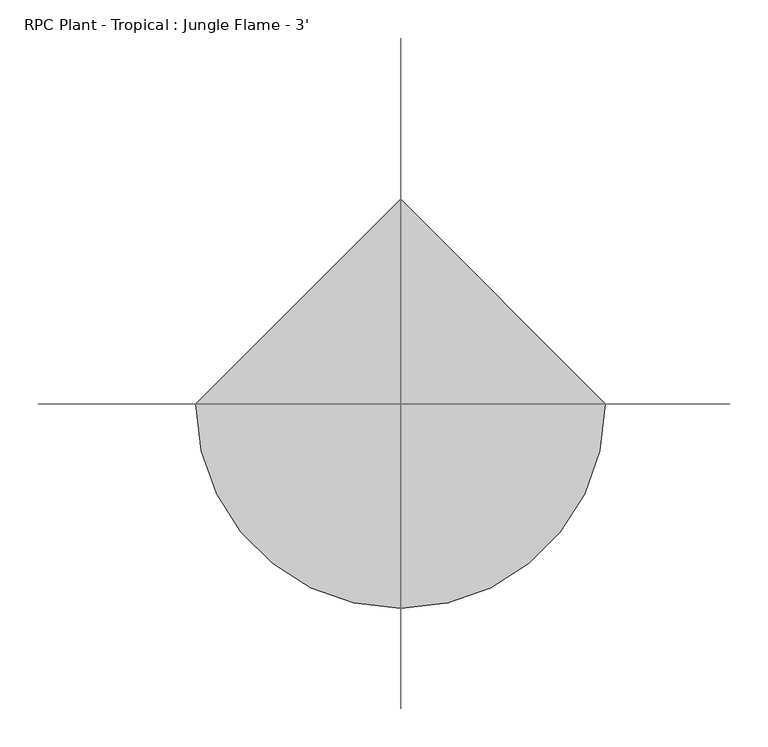
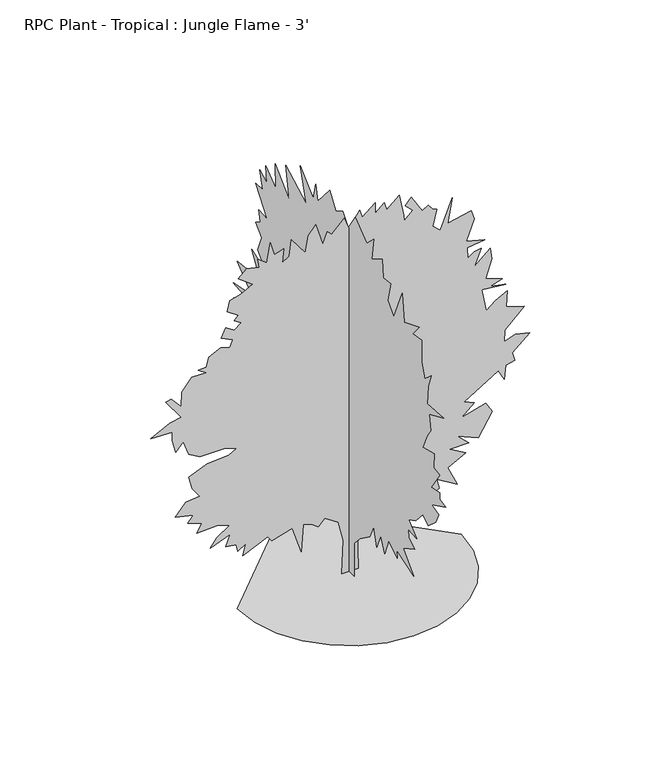
"""IFC4 building model written with IfcOpenShell, lengths in millimetres: geographic element geometry, RPC Plant - Tropical : Jungle Flame - 3'."""

from ifc_helpers import new_model, si_unit, origin, place, context, project, spatial, triangles, source, transform, mapped, element, save


def rpc_plant_tropical_jungle_flame_3_9c4808c2(model_context):
    return source(origin(), model_context, "Body", "Tessellation", [
        triangles([(-268.0952273, 0.0, 4.64e-05), (-261.0086141, -61.4296216, 4.64e-05), (-240.8232365, -117.8430704, 4.64e-05), (-209.155511, -167.6236892, 4.64e-05), (-167.6236892, -209.1557472, 4.64e-05), (-117.8430704, -240.8232365, 4.64e-05), (-61.4296216, -261.0086141, 4.64e-05), (1.17e-05, -268.0952273, 4.64e-05), (61.4296216, -261.0086141, 4.64e-05), (117.8430704, -240.8232365, 4.64e-05), (167.6236892, -209.155511, 4.64e-05), (209.1557472, -167.6236892, 4.64e-05), (240.8232365, -117.8430704, 4.64e-05), (261.0086141, -61.4296216, 4.64e-05), (268.0952273, 2.34e-05, 4.64e-05), (-3.52e-05, 268.0952273, 4.64e-05), (-1.48e-05, -20.1101483, 4.49e-05), (-1.23e-05, -20.1680527, 84.1033148), (-1.26e-05, -43.4307974, 109.1553558), (-1.36e-05, -84.5877148, 139.5758464), (-1.33e-05, -102.4820622, 175.3643141), (-1.52e-05, -115.0079782, 130.6286726), (-1.47e-05, -131.1128455, 169.9961098), (-1.65e-05, -147.2177128, 134.2074059), (-1.6e-05, -163.3225891, 177.1537943), (-1.83e-05, -199.111284, 153.8912426), (-1.76e-05, -197.3218038, 173.5750701), (-2.14e-05, -267.1099495, 150.3122731), (-1.81e-05, -224.163334, 195.0481417), (-1.95e-05, -270.6875473, 220.1001918), (-1.79e-05, -245.6375502, 234.4155789), (-1.73e-05, -243.8476158, 254.100333), (-1.89e-05, -279.6349481, 252.3103987), (-1.66e-05, -247.4252136, 280.9402645), (-1.75e-05, -276.0573685, 295.2574684), (-1.78e-05, -304.6872162, 327.4672211), (-1.92e-05, -327.9495681, 314.9399334), (-1.98e-05, -358.3716574, 341.782154), (-1.95e-05, -370.8966559, 368.6220855), (-1.8e-05, -342.2667901, 375.7818229), (-1.97e-05, -399.5287745, 404.4116887), (-1.85e-05, -374.4765246, 409.7792027), (-1.8e-05, -374.4765246, 425.8840699), (-1.67e-05, -340.4768558, 418.7266216), (-1.67e-05, -374.4765246, 470.6210921), (-1.54e-05, -349.4242384, 474.1987081), (-1.44e-05, -351.2141727, 509.9883113), (-1.27e-05, -304.6872162, 499.250958), (-1.23e-05, -322.5820178, 538.6181771), (-1.23e-05, -336.8969507, 560.0928474), (-1.09e-05, -331.5294368, 597.6701323), (-1.28e-05, -390.5813919, 624.5123165), (-9.9e-06, -322.5820178, 619.1448389), (-8.7e-06, -327.9495681, 667.4594044), (-8.2e-06, -338.6868851, 699.6691389), (-7.7e-06, -311.8447008, 676.4045706), (-6.1e-06, -299.3197022, 710.4042395), (-4.5e-06, -299.3197022, 765.8762896), (-3.1e-06, -263.5300808, 760.5087393), (-3.3e-06, -290.3722833, 792.7184738), (-1.2e-06, -227.7422944, 767.6662239), (1.2e-06, -218.7951116, 835.6655617), (3e-07, -184.7958969, 755.1412617), (2.2e-06, -159.7438468, 781.9811932), (3.2e-06, -172.2697537, 832.085693), (4.4e-06, -141.8494994, 828.5081497), (5.9e-06, -136.4810589, 871.4529121), (7.1e-06, -93.5348885, 846.4006622), (8.4e-06, -100.692582, 900.0851034), (8.9e-06, -72.0615762, 873.2428465), (1.21e-05, -25.5364477, 910.8201313), (1.2e-05, 3.0945581, 866.0853619), (1.39e-05, 26.3571235, 894.7152277), (1.47e-05, 54.9881316, 878.6103968), (1.69e-05, 80.0401726, 914.4), (1.74e-05, 130.1442636, 857.1380156), (1.89e-05, 139.0914373, 894.7152277), (1.81e-05, 149.8281003, 851.7704653), (2.2e-05, 203.5109246, 901.8750378), (1.85e-05, 178.4588745, 821.3506651), (2.37e-05, 262.5630977, 867.8752962), (2.07e-05, 248.2458757, 789.1409306), (2.49e-05, 305.5079146, 844.6129807), (2.3e-05, 303.7202512, 783.7711275), (2.58e-05, 344.8750975, 815.980862), (2.44e-05, 341.2975179, 774.8237085), (2.62e-05, 369.9273837, 790.9285395), (2.43e-05, 357.4023851, 747.983777), (2.56e-05, 387.8221853, 746.1938427), (2.16e-05, 339.5075835, 683.564308), (2.32e-05, 373.5072524, 687.1418512), (2.22e-05, 368.1397385, 660.299667), (2.27e-05, 387.8221853, 647.7747047), (2.08e-05, 362.7698991, 622.7223822), (2.04e-05, 378.8747663, 583.3551993), (1.77e-05, 343.0874522, 547.5655961), (2.11e-05, 403.9270526, 569.0402664), (1.71e-05, 360.9799647, 499.250958), (1.89e-05, 393.1896993, 511.7782456), (2.17e-05, 462.9790077, 502.830863), (1.77e-05, 403.9270526, 454.5162249), (2.05e-05, 479.083875, 438.4113576), (1.67e-05, 396.7696043, 431.2539093), (1.57e-05, 387.8221853, 411.569137), (1.94e-05, 477.2939406, 402.6217544), (1.5e-05, 394.97967, 377.5694681), (1.44e-05, 411.0845372, 332.834735), (1.36e-05, 368.1397385, 370.4120198), (1.19e-05, 355.6124508, 334.6246694), (1.33e-05, 398.5595387, 314.9399334), (1.21e-05, 400.349473, 271.9928455), (8.7e-06, 341.2975179, 248.7305118), (1.01e-05, 384.2446057, 229.0480649), (4.9e-06, 291.1929636, 195.0481417), (6.5e-06, 341.2975179, 175.3643141), (6.7e-06, 369.9273837, 135.996886), (4.2e-06, 294.7728504, 166.4173675), (2.6e-06, 289.4030292, 121.6814898), (2.3e-06, 258.983229, 157.4702029), (0.0, 239.300764, 107.3661027), (1.6e-06, 241.0884092, 159.2594469), (1.2e-06, 228.5629746, 164.6278873), (-1.1e-06, 203.5109246, 127.0497123), (-2e-07, 205.3004047, 153.8912426), (-1.9e-06, 162.3540072, 159.2594469), (-2.4e-06, 167.7222116, 135.996886), (-3e-06, 139.0914373, 157.4702029), (-5.5e-06, 130.1442636, 89.4717553), (-5.5e-06, 74.6719592, 171.78559), (-6.4e-06, 62.1458251, 161.048927), (-7.4e-06, 37.0937796, 164.6278873), (-7.6e-06, 51.4093984, 134.2074059), (-8.5e-06, 15.6205809, 157.4702029), (-1.29e-05, 22.7783675, 4.61e-05), (-17.334692, 5.3e-05, 1.7e-06), (-13.7758477, 4.79e-05, 83.6317139), (-26.2316224, 4.54e-05, 133.4546266), (-58.2607652, 4.56e-05, 154.8074657), (-74.27534, 4.72e-05, 138.7928909), (-90.2899103, 4.72e-05, 151.2486168), (-109.863334, 4.77e-05, 156.5868811), (-115.2013712, 5.19e-05, 90.7491664), (-136.5542103, 4.89e-05, 156.5868811), (-184.5979257, 5.18e-05, 142.3517307), (-195.2742362, 5.15e-05, 156.5868811), (-253.9951796, 5.57e-05, 128.1165803), (-246.8765734, 5.37e-05, 156.5868811), (-266.4493067, 5.53e-05, 144.1311552), (-270.0086098, 5.44e-05, 161.9249273), (-294.9214242, 5.53e-05, 165.4837762), (-284.2435331, 5.31e-05, 193.954077), (-332.2884021, 5.64e-05, 174.3808894), (-316.2726645, 5.44e-05, 195.7334923), (-286.024311, 5.18e-05, 217.0863314), (-316.2726645, 5.26e-05, 225.9832084), (-364.3175517, 5.48e-05, 224.203793), (-351.8611173, 5.31e-05, 243.7767626), (-385.6687921, 5.38e-05, 256.2331607), (-373.2146467, 5.23e-05, 272.2465909), (-415.9194165, 5.36e-05, 282.9245002), (-391.0088731, 5.08e-05, 311.3943649), (-357.1989455, 4.91e-05, 314.953668), (-374.9931719, 4.84e-05, 339.8641751), (-383.8902669, 4.69e-05, 371.8933248), (-339.4047192, 4.38e-05, 391.4660763), (-287.8028362, 4.13e-05, 395.0253794), (-268.2301028, 3.98e-05, 405.7032887), (-300.2592343, 4.07e-05, 414.5980946), (-357.1989455, 4.32e-05, 414.5980946), (-383.8902669, 4.34e-05, 430.6138321), (-396.346665, 4.18e-05, 466.2022848), (-414.1408914, 4.37e-05, 446.6272442), (-423.0357336, 4.22e-05, 478.6563938), (-423.0357336, 4.09e-05, 500.0099233), (-474.6398875, 4.31e-05, 501.7884121), (-428.3758146, 3.97e-05, 524.9227558), (-401.6844933, 3.82e-05, 530.2605477), (-439.0514348, 3.68e-05, 581.8624489), (-424.8165115, 3.6e-05, 583.6409377), (-401.6844933, 3.66e-05, 556.9519054), (-399.903679, 3.44e-05, 592.5380691), (-376.7716607, 3.16e-05, 622.7887299), (-341.1854971, 3.02e-05, 621.0078793), (-360.7582486, 3.02e-05, 635.2450916), (-341.1854971, 2.93e-05, 635.2450916), (-335.8454161, 2.77e-05, 658.3771099), (-307.3755695, 2.56e-05, 672.6120695), (-286.024311, 2.51e-05, 665.4934633), (-278.905723, 2.37e-05, 683.2876534), (-305.5970444, 2.41e-05, 695.7440878), (-294.9214242, 2.23e-05, 718.8761061), (-275.3464199, 2.22e-05, 706.4197443), (-257.5521935, 2.07e-05, 718.8761061), (-275.3464199, 2.08e-05, 729.5517626), (-264.6707997, 1.97e-05, 740.2273464), (-291.3621211, 1.98e-05, 758.0216091), (-286.024311, 1.8e-05, 784.7129305), (-259.3329896, 1.64e-05, 791.8315367), (-230.8631431, 1.43e-05, 806.0664963), (-264.6707997, 1.42e-05, 832.7578176), (-245.0980664, 1.23e-05, 850.5520077), (-214.8476599, 1.14e-05, 843.4334015), (-218.4062726, 1.03e-05, 864.7869673), (-197.0536516, 1.03e-05, 848.7712297), (-188.1565384, 7e-06, 896.8161169), (-179.2596614, 8.7e-06, 863.0061167), (-156.1274069, 7.2e-06, 870.1247229), (-159.6862377, 9.4e-06, 836.3147953), (-143.6716719, 8.1e-06, 846.9927046), (-138.3334077, 5.5e-06, 886.1382076), (-104.5250607, 6.7e-06, 841.6548763), (-97.407372, 3.9e-06, 882.5811573), (-79.6133818, 1.9e-06, 903.9323977), (-63.599034, 4.4e-06, 848.7712297), (-52.922501, 2.3e-06, 877.2410763), (-42.246195, 2.5e-06, 866.5654198), (-11.9964482, -7e-07, 896.8161169), (-1.3200484, 6e-07, 868.3439449), (25.3709418, -2.7e-06, 903.9323977), (30.7089813, -1.8e-06, 884.3596825), (62.7381264, -4.7e-06, 909.2702259), (62.7381264, -3.1e-06, 882.5811573), (84.09097, -5.2e-06, 902.1538725), (89.4290072, -4.3e-06, 882.5811573), (119.6787324, -7.2e-06, 909.2702259), (130.3552609, -4.4e-06, 854.109058), (132.1346854, -3.6e-06, 839.8740984), (151.7078729, -5.6e-06, 859.449139), (133.9138827, -5.9e-06, 877.2410763), (148.1492602, -7.5e-06, 893.2568138), (174.8401455, -6.1e-06, 850.5520077), (189.0752868, -7.2e-06, 859.449139), (197.9721638, -6.9e-06, 846.9927046), (208.6487105, -7e-06, 841.6548763), (199.7515974, -4.3e-06, 802.5071932), (217.5455875, -4.1e-06, 786.4937084), (246.0147437, -9.6e-06, 857.6683611), (235.3391235, -5.5e-06, 797.1693649), (292.2811057, -8.8e-06, 809.6257267), (299.3974228, -7.7e-06, 786.4937084), (279.8246894, -3.9e-06, 736.6703688), (324.3102553, -5.1e-06, 724.2139343), (281.6031964, -2.9e-06, 718.8761061), (283.3839925, -1.4e-06, 692.1847847), (299.3974228, -2.7e-06, 702.8604412), (315.413124, -3.6e-06, 706.4197443), (299.3974228, -5e-07, 665.4934633), (336.7643643, -4.1e-06, 699.3033909), (340.3236674, -2.6e-06, 670.8312916), (326.0887442, 7e-07, 626.348033), (365.2365, -2e-07, 612.1130733), (336.7643643, 1.6e-06, 603.2159783), (374.1313422, 5e-07, 594.318847), (317.1916492, 2.5e-06, 601.4351641), (327.8672693, 5.5e-06, 544.495471), (349.2207988, 3.5e-06, 562.2896974), (377.6906453, 1.4e-06, 576.5246206), (375.9121202, 3.8e-06, 537.3768648), (418.61689, 2.8e-06, 523.1419415), (372.3528171, 7.4e-06, 478.6563938), (370.5743282, 9.2e-06, 450.1865473), (397.2633605, 7.4e-06, 460.8644566), (431.0732881, 6.5e-06, 451.9673615), (390.1470434, 1.04e-05, 416.3789088), (395.4848717, 1.14e-05, 395.0253794), (374.1313422, 1.27e-05, 389.6875511), (370.5743282, 1.48e-05, 355.8799127), (356.339405, 1.39e-05, 382.5689449), (274.4868793, 2.04e-05, 332.747858), (299.3974228, 2e-05, 322.0699851), (267.3682732, 2.3e-05, 295.3786274), (326.0887442, 1.94e-05, 311.3943649), (342.1021926, 2.03e-05, 284.7030072), (308.2945178, 2.51e-05, 229.5418393), (258.47116, 2.6e-05, 250.8953506), (285.1624995, 2.63e-05, 225.9832084), (240.6769336, 2.84e-05, 224.203793), (278.0438933, 2.8e-05, 202.8511901), (235.3391235, 3.13e-05, 179.7189175), (258.47116, 3.32e-05, 129.8957777), (208.6484744, 3.36e-05, 160.1454938), (215.7661722, 3.48e-05, 135.234042), (180.1781736, 3.73e-05, 119.2194762), (146.3698357, 3.69e-05, 149.4691923), (151.7078729, 4.11e-05, 76.5140161), (132.1346854, 3.8e-05, 142.3517307), (82.3115456, 4.26e-05, 101.425477), (91.2084316, 3.97e-05, 144.1311552), (53.8412448, 4.43e-05, 94.3080153), (43.1647072, 4.28e-05, 126.337165), (66.2969707, 3.83e-05, 185.0571818), (34.2678257, 4e-05, 179.7189175), (18.2532304, 4.23e-05, 153.0280322), (21.8120066, 5.13e-05, 0.0)], [[15, 16, 1], [14, 15, 1], [14, 1, 2], [13, 14, 2], [13, 2, 3], [13, 3, 4], [12, 13, 4], [11, 12, 4], [11, 4, 5], [11, 5, 6], [11, 6, 7], [11, 7, 8], [11, 8, 9], [11, 9, 10], [101, 102, 103], [119, 120, 121], [51, 52, 53], [104, 105, 106], [76, 77, 78], [27, 28, 29], [59, 60, 61], [106, 107, 108], [78, 79, 80], [122, 123, 124], [61, 62, 63], [54, 55, 56], [131, 132, 133], [115, 116, 117], [114, 115, 117], [21, 22, 23], [40, 41, 42], [32, 33, 34], [96, 97, 98], [68, 69, 70], [125, 126, 127], [127, 128, 129], [82, 83, 84], [86, 87, 88], [112, 113, 114], [23, 24, 25], [99, 100, 101], [84, 85, 86], [117, 118, 119], [80, 81, 82], [25, 26, 27], [88, 89, 90], [29, 30, 31], [44, 45, 46], [66, 67, 68], [64, 65, 66], [90, 91, 92], [46, 47, 48], [74, 75, 76], [92, 93, 94], [42, 43, 44], [40, 42, 44], [38, 39, 40], [98, 99, 101], [57, 58, 59], [70, 71, 72], [133, 134, 17], [133, 17, 18], [133, 18, 19], [104, 106, 108], [114, 117, 119], [72, 73, 74], [133, 19, 20], [37, 38, 40], [36, 37, 40], [133, 20, 21], [110, 111, 112], [109, 110, 112], [44, 46, 48], [53, 54, 56], [94, 95, 96], [98, 101, 103], [90, 92, 94], [68, 70, 72], [114, 119, 121], [114, 121, 122], [98, 103, 104], [129, 130, 131], [64, 66, 68], [86, 88, 90], [84, 86, 90], [82, 84, 90], [25, 27, 29], [25, 29, 31], [25, 31, 32], [57, 59, 61], [57, 61, 63], [56, 57, 63], [53, 56, 63], [98, 104, 108], [49, 50, 51], [36, 40, 44], [36, 44, 48], [35, 36, 48], [34, 35, 48], [25, 32, 34], [23, 25, 34], [21, 23, 34], [21, 34, 48], [133, 21, 48], [131, 133, 48], [129, 131, 48], [90, 94, 96], [82, 90, 96], [80, 82, 96], [109, 112, 114], [109, 114, 122], [64, 68, 72], [122, 124, 125], [109, 122, 125], [109, 125, 127], [109, 127, 129], [109, 129, 48], [108, 109, 48], [98, 108, 48], [96, 98, 48], [80, 96, 48], [78, 80, 48], [76, 78, 48], [74, 76, 48], [72, 74, 48], [64, 72, 48], [63, 64, 48], [53, 63, 48], [53, 48, 49], [53, 49, 51], [252, 253, 254], [236, 237, 238], [284, 285, 286], [141, 142, 143], [241, 242, 243], [204, 205, 206], [174, 175, 176], [151, 152, 153], [279, 280, 281], [266, 267, 268], [183, 184, 185], [250, 251, 252], [151, 153, 154], [286, 287, 288], [202, 203, 204], [209, 210, 211], [275, 276, 277], [145, 146, 147], [218, 219, 220], [220, 221, 222], [247, 248, 249], [288, 289, 290], [288, 290, 291], [155, 156, 157], [262, 263, 264], [212, 213, 214], [211, 212, 214], [245, 246, 247], [244, 245, 247], [171, 172, 173], [277, 278, 279], [261, 262, 264], [224, 225, 226], [256, 257, 258], [177, 178, 179], [177, 179, 180], [258, 259, 260], [222, 223, 224], [159, 160, 161], [269, 270, 271], [247, 249, 250], [216, 217, 218], [214, 215, 216], [206, 207, 208], [147, 148, 149], [250, 252, 254], [159, 161, 162], [157, 158, 159], [229, 230, 231], [228, 229, 231], [193, 194, 195], [149, 150, 151], [199, 200, 201], [199, 201, 202], [190, 191, 192], [189, 190, 192], [294, 135, 136], [293, 294, 136], [293, 136, 137], [204, 206, 208], [174, 176, 177], [264, 265, 266], [231, 232, 233], [238, 239, 240], [238, 240, 241], [236, 238, 241], [138, 139, 140], [255, 256, 258], [255, 258, 260], [163, 164, 165], [281, 282, 283], [281, 283, 284], [273, 274, 275], [272, 273, 275], [271, 272, 275], [233, 234, 235], [231, 233, 235], [162, 163, 165], [162, 165, 166], [143, 144, 145], [195, 196, 197], [195, 197, 198], [227, 228, 231], [227, 231, 235], [171, 173, 174], [171, 174, 177], [261, 264, 266], [261, 266, 268], [195, 198, 199], [293, 137, 138], [292, 293, 138], [157, 159, 162], [155, 157, 162], [155, 162, 166], [154, 155, 166], [154, 166, 167], [286, 288, 291], [284, 286, 291], [181, 182, 183], [180, 181, 183], [247, 250, 254], [147, 149, 151], [185, 186, 187], [185, 187, 188], [183, 185, 188], [199, 202, 204], [199, 204, 208], [224, 226, 227], [277, 279, 281], [277, 281, 284], [277, 284, 291], [261, 268, 269], [189, 192, 193], [236, 241, 243], [193, 195, 199], [193, 199, 208], [145, 147, 151], [145, 151, 154], [145, 154, 167], [143, 145, 167], [141, 143, 167], [222, 224, 227], [275, 277, 291], [271, 275, 291], [269, 271, 291], [177, 180, 183], [140, 141, 167], [138, 140, 167], [292, 138, 167], [291, 292, 167], [269, 291, 167], [261, 269, 167], [260, 261, 167], [255, 260, 167], [254, 255, 167], [247, 254, 167], [244, 247, 167], [243, 244, 167], [236, 243, 167], [235, 236, 167], [227, 235, 167], [222, 227, 167], [220, 222, 167], [218, 220, 167], [216, 218, 167], [214, 216, 167], [211, 214, 167], [209, 211, 167], [208, 209, 167], [193, 208, 167], [189, 193, 167], [188, 189, 167], [183, 188, 167], [177, 183, 167], [177, 167, 168], [171, 177, 168], [171, 168, 169], [170, 171, 169]], closed=False),
    ])


if __name__ == "__main__":
    model = new_model("IFC4")
    model_context = context("Model", 3, world=origin())
    ifc_project = project(units=[si_unit("LENGTHUNIT", "METRE", prefix="MILLI")], contexts=[model_context])
    site = spatial("IfcSite", under=ifc_project)
    building = spatial("IfcBuilding", under=site)
    placement = place(None, origin())
    rpc_plant_tropical_jungle_flame_3_shape = rpc_plant_tropical_jungle_flame_3_9c4808c2(model_context)
    element("IfcGeographicElement", 1, ObjectType="RPC Plant - Tropical : Jungle Flame - 3'", at=placement, inside=building, context=model_context, shape_type="MappedRepresentation", body=[
        mapped(rpc_plant_tropical_jungle_flame_3_shape, transform((0.0, 0.0, 0.0), x_axis=(1.0, 0.0, 0.0), y_axis=(0.0, 1.0, 0.0), z_axis=(0.0, 0.0, 1.0))),
    ])
    save(model, "model.ifc")

# Revit data of these elements
# Type "RPC Plant - Tropical : Jungle Flame - 3'"
#   built-in parameter 1005198 = "{2, 15},{39, RPC-16-FUVJ-JWG0-MWGK-8000-ST1L-LVER-AU},{1, 0},{1, 0},{2, 13},{1, 8},{5, Color},{1, 0},{1, 0},{3, 0.8},{3, 0.8},{3, 0.8},{1, 8},{7, BBoxMin},{1, 0},{1, 0},{1, 0},{1, 0},{1, 0},{1, 8},{7, BBoxMax},{1, 0},{1, 0},{1, 0},{1, 0},{1, 0},{2, 11},{9, RPCTypeId},{1, 0},{1, 0},{39, RPC-16-FUVJ-JWG0-MWGK-8000-ST1L-LVER-AU},{1, 6},{14, RPCPlantHeight},{1, 0},{1, 0},{1, 3},{2, 11},{7, keyword},{1, 0},{1, 0},{35, :RPCs:Shrubs [General]:Geometry:RPC},{2, 11},{8, category},{1, 0},{1, 0},{16, Shrubs [General]},{2, 11},{12, LocalizedUID},{1, 0},{1, 0},{12, Jungle Flame},{2, 14},{6, Height},{1, 0},{1, 0},{1, 3},{1, 2},{16, Cast Reflections},{1, 0},{1, 0},{1, 0},{1, 2},{12, Cast Shadows},{1, 0},{1, 0},{1, 1},{1, 2},{9, Lock View},{1, 0},{1, 0},{1, 0},{1, 4},{5, ViewC},{1, 0},{1, 0},{1, 0},{21, assetlibrary_base.fbx},{1, 5},"
#   built-in parameter 1005195 = "RPC-16-FUVJ-JWG0-MWGK-8000-ST1L-LVER-AU"
#   Type Comments = "Jungle Flame"
#   Assembly Code = "G2050500"
#   Height = 3' - 0"
#   Default Elevation = 0
